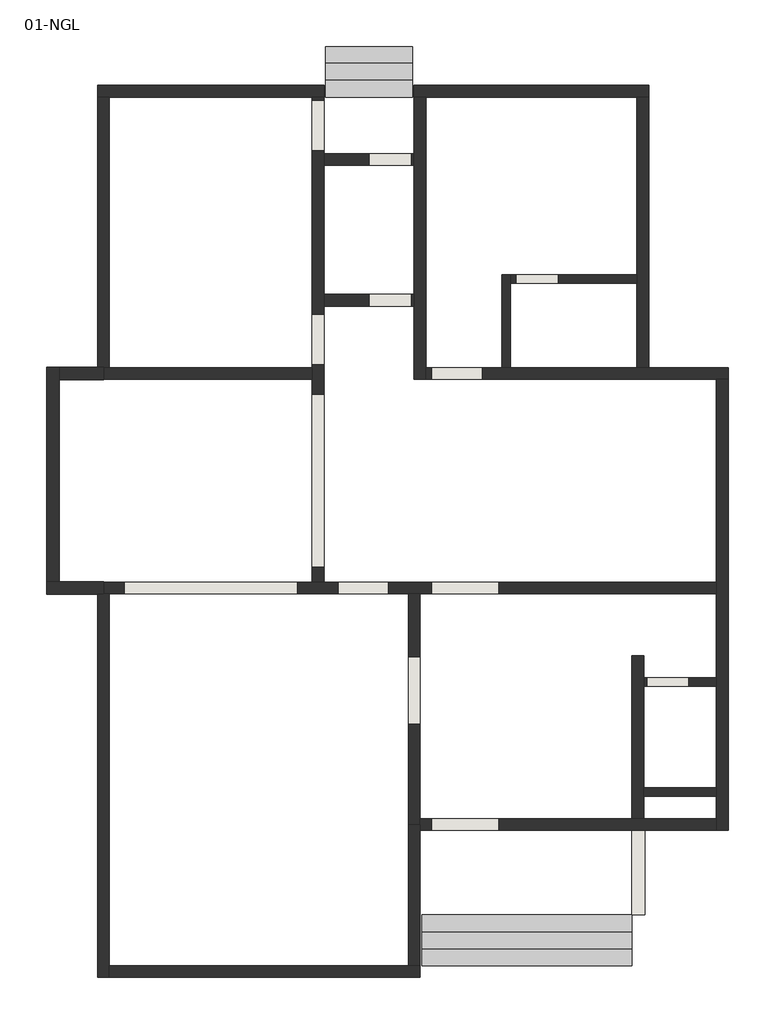
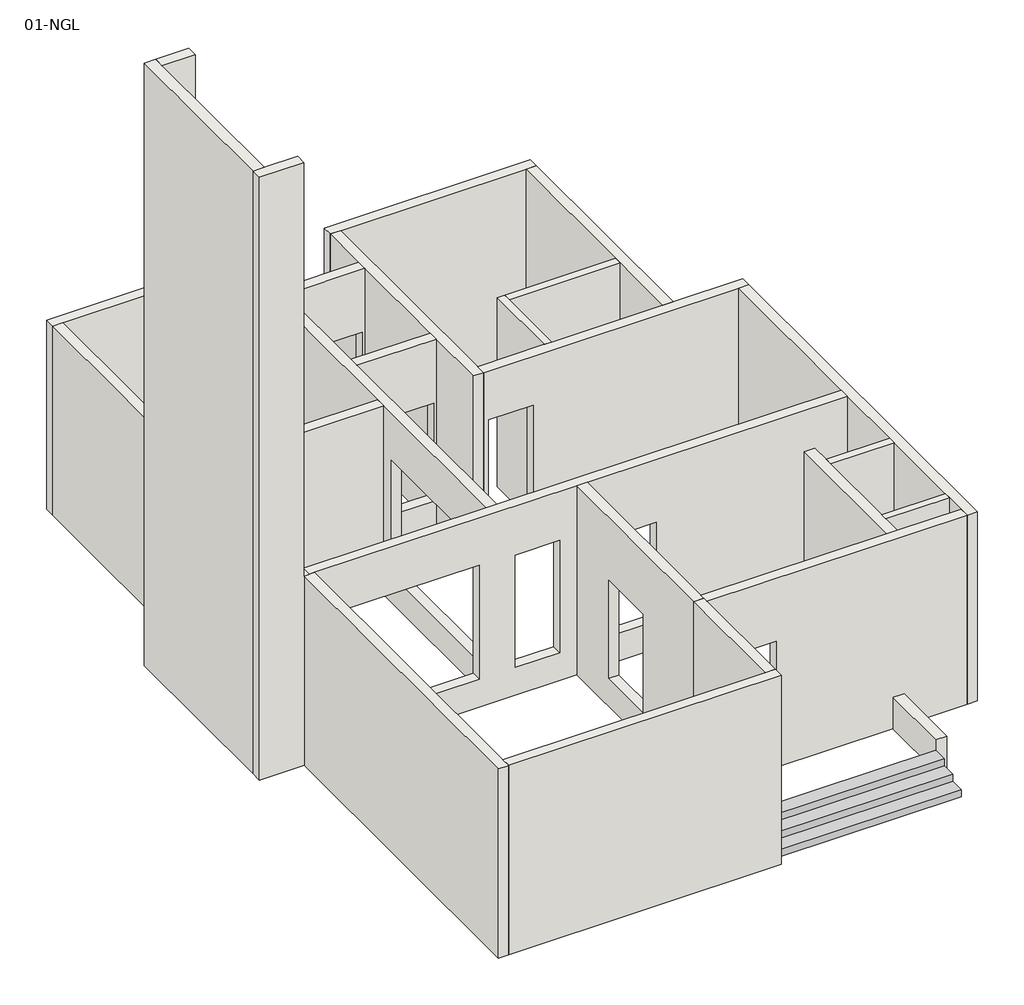
# One storey: 26 walls, 2 stair flights.
"""IFC4 building model written with IfcOpenShell, lengths in millimetres."""

from ifc_helpers import new_model, si_unit, frame, origin, origin_with_axes, place, context, project, spatial, polyline, outline, extrude, faceted_brep, element, save

model = new_model("IFC4")

# Units and contexts
model_context = context("Model", 3, world=origin())
ifc_project = project(units=[si_unit("LENGTHUNIT", "METRE", prefix="MILLI")], contexts=[model_context])

# Site, building, storey
site = spatial("IfcSite", under=ifc_project)
building = spatial("IfcBuilding", under=site)
storey = spatial("IfcBuildingStorey", under=building, Name="01-NGL", Elevation=0.0)

# Stair flights
placement = place(None, origin())
element("IfcStairFlight", 1, ObjectType="00-STEPS", at=placement, inside=storey, context=model_context, shape_type="Brep", body=[
    faceted_brep([(-8789.1107921, -18814.8987034, 150.0), (-8789.1107921, -19114.8987034, 150.0), (-5054.1107921, -19114.8987034, 150.0), (-5054.1107921, -18814.8987034, 150.0), (-8789.1107921, -18814.8987034, 0.0), (-8789.1107921, -19114.8987034, 0.0), (-5054.1107921, -19114.8987034, 0.0), (-5054.1107921, -18814.8987034, 0.0), (-8789.1107921, -18514.8987034, 300.0), (-8789.1107921, -18814.8987034, 300.0), (-5054.1107921, -18814.8987034, 300.0), (-5054.1107921, -18514.8987034, 300.0), (-8789.1107921, -18514.8987034, 0.0), (-5054.1107921, -18514.8987034, 0.0), (-8789.1107921, -18214.8987034, 0.0), (-5054.1107921, -18214.8987034, 0.0), (-8789.1107921, -18214.8987034, 450.0), (-8789.1107921, -18514.8987034, 450.0), (-5054.1107921, -18514.8987034, 450.0), (-5054.1107921, -18214.8987034, 450.0)], [[[0, 1, 2, 3]], [[1, 0, 4, 5]], [[2, 1, 5, 6]], [[3, 2, 6, 7]], [[8, 9, 10, 11]], [[4, 0, 9, 8, 12]], [[0, 3, 10, 9]], [[3, 7, 13, 11, 10]], [[5, 4, 12, 14, 15, 13, 7, 6]], [[16, 17, 18, 19]], [[12, 8, 17, 16, 14]], [[8, 11, 18, 17]], [[11, 13, 15, 19, 18]], [[16, 19, 15, 14]]]),
])
element("IfcStairFlight", 2, ObjectType="00-STEPS", at=placement, inside=storey, context=model_context, shape_type="Brep", body=[
    faceted_brep([(-8954.1107921, -3094.8987034, 150.0), (-8954.1107921, -2794.8987034, 150.0), (-10499.1107921, -2794.8987034, 150.0), (-10499.1107921, -3094.8987034, 150.0), (-8954.1107921, -3094.8987034, 0.0), (-8954.1107921, -2794.8987034, 0.0), (-10499.1107921, -2794.8987034, 0.0), (-10499.1107921, -3094.8987034, 0.0), (-8954.1107921, -3394.8987034, 300.0), (-8954.1107921, -3094.8987034, 300.0), (-10499.1107921, -3094.8987034, 300.0), (-10499.1107921, -3394.8987034, 300.0), (-8954.1107921, -3394.8987034, 0.0), (-10499.1107921, -3394.8987034, 0.0), (-8954.1107921, -3694.8987034, 0.0), (-10499.1107921, -3694.8987034, 0.0), (-8954.1107921, -3694.8987034, 450.0), (-8954.1107921, -3394.8987034, 450.0), (-10499.1107921, -3394.8987034, 450.0), (-10499.1107921, -3694.8987034, 450.0)], [[[0, 1, 2, 3]], [[1, 0, 4, 5]], [[2, 1, 5, 6]], [[3, 2, 6, 7]], [[8, 9, 10, 11]], [[4, 0, 9, 8, 12]], [[0, 3, 10, 9]], [[3, 7, 13, 11, 10]], [[5, 4, 12, 14, 15, 13, 7, 6]], [[16, 17, 18, 19]], [[12, 8, 17, 16, 14]], [[8, 11, 18, 17]], [[11, 13, 15, 19, 18]], [[16, 19, 15, 14]]]),
])

# Walls
element("IfcWall", 3, ObjectType="00 BRICK WALL", at=placement, inside=storey, context=model_context, shape_type="Brep", body=[
    faceted_brep([(-15456.6107921, -8487.3987034, 0.0), (-15456.6107921, -12297.3987034, 0.0), (-15456.6107921, -12297.3987034, 12900.0), (-15456.6107921, -8487.3987034, 12900.0), (-15231.6107921, -8487.3987034, 0.0), (-15231.6107921, -8487.3987034, 12900.0), (-15231.6107921, -8712.3987034, 12900.0), (-15231.6107921, -12297.3987034, 12900.0), (-15231.6107921, -12297.3987034, 0.0), (-15231.6107921, -8712.3987034, 0.0)], [[[0, 1, 2, 3]], [[4, 5, 6, 7, 8, 9]], [[1, 0, 4, 9, 8]], [[3, 2, 7, 6, 5]], [[0, 3, 5, 4]], [[2, 1, 8, 7]]]),
])
element("IfcWall", 4, ObjectType="00 BRICK WALL", at=placement, inside=storey, context=model_context, shape_type="Brep", body=[
    faceted_brep([(-14444.1107921, -12297.3987034, 4050.0), (-14444.1107921, -12297.3987034, 0.0), (-15231.6107921, -12297.3987034, 0.0), (-15456.6107921, -12297.3987034, 0.0), (-15456.6107921, -12297.3987034, 12900.0), (-15231.6107921, -12297.3987034, 12900.0), (-14556.6107921, -12297.3987034, 12900.0), (-14556.6107921, -12297.3987034, 4050.0), (-14444.1107921, -12522.3987034, 0.0), (-14444.1107921, -12522.3987034, 4050.0), (-14549.1107921, -12522.3987034, 4050.0), (-14556.6107921, -12522.3987034, 4050.0), (-14556.6107921, -12522.3987034, 7500.0), (-14556.6107921, -12522.3987034, 12900.0), (-15456.6107921, -12522.3987034, 12900.0), (-15456.6107921, -12522.3987034, 0.0), (-14549.1107921, -12522.3987034, 0.0), (-14444.1107921, -12304.8987034, 0.0), (-14444.1107921, -12514.8987034, 0.0), (-14444.1107921, -12304.8987034, 4050.0), (-14444.1107921, -12514.8987034, 4050.0), (-14556.6107921, -12299.8987034, 4050.0)], [[[0, 1, 2, 3, 4, 5, 6, 7]], [[8, 9, 10, 11, 12, 13, 14, 15, 16]], [[3, 2, 1, 17, 18, 8, 16, 15]], [[6, 5, 4, 14, 13]], [[4, 3, 15, 14]], [[0, 19, 20, 9, 8, 18, 17, 1]], [[7, 21, 11, 10, 9, 20, 19, 0]], [[6, 13, 12, 11, 21, 7]]]),
])
element("IfcWall", 5, ObjectType="00 BRICK WALL", at=placement, inside=storey, context=model_context, shape_type="Brep", body=[
    faceted_brep([(-14444.1107921, -8487.3987034, 0.0), (-14549.1107921, -8487.3987034, 0.0), (-15231.6107921, -8487.3987034, 0.0), (-15231.6107921, -8487.3987034, 12900.0), (-14556.6107921, -8487.3987034, 12900.0), (-14556.6107921, -8487.3987034, 4050.0), (-14549.1107921, -8487.3987034, 4050.0), (-14444.1107921, -8487.3987034, 4050.0), (-14444.1107921, -8712.3987034, 0.0), (-14444.1107921, -8712.3987034, 4050.0), (-14556.6107921, -8712.3987034, 4050.0), (-14556.6107921, -8712.3987034, 7575.0), (-14556.6107921, -8712.3987034, 12900.0), (-15231.6107921, -8712.3987034, 12900.0), (-15231.6107921, -8712.3987034, 0.0), (-14444.1107921, -8494.8987034, 0.0), (-14444.1107921, -8704.8987034, 0.0), (-14444.1107921, -8494.8987034, 4050.0), (-14444.1107921, -8704.8987034, 4050.0)], [[[0, 1, 2, 3, 4, 5, 6, 7]], [[8, 9, 10, 11, 12, 13, 14]], [[2, 1, 0, 15, 16, 8, 14]], [[4, 3, 13, 12]], [[3, 2, 14, 13]], [[0, 7, 17, 18, 9, 8, 16, 15]], [[5, 10, 9, 18, 17, 7, 6]], [[5, 4, 12, 11, 10]]]),
])
element("IfcWall", 6, ObjectType="01-150 WALL", at=placement, inside=storey, context=model_context, shape_type="SweptSolid", body=[
    extrude(outline(polyline([(-3554.1107921, -16104.8987034), (-4844.1107921, -16104.8987034), (-4844.1107921, -15954.8987034), (-3554.1107921, -15954.8987034), (-3554.1107921, -16104.8987034)])), origin_with_axes(), (0.0, 0.0, 1.0), 4050.0),
])
element("IfcWall", 7, ObjectType="01-150 WALL", at=placement, inside=storey, context=model_context, shape_type="SweptSolid", body=[
    extrude(outline(polyline([(0.0, -4844.1107921), (0.0, -3554.1107921), (4050.0, -3554.1107921), (4050.0, -4844.1107921), (0.0, -4844.1107921)]), holes=[polyline([(600.0, -4794.1107921), (2700.0, -4794.1107921), (2700.0, -4044.1107921), (600.0, -4044.1107921), (600.0, -4794.1107921)])]), frame((0.0, -14154.8987034, 0.0), z_axis=(0.0, 1.0, 0.0), x_axis=(0.0, 0.0, 1.0)), (0.0, 0.0, 1.0), 150.0),
])
element("IfcWall", 8, ObjectType="01-150 WALL", at=placement, inside=storey, context=model_context, shape_type="Brep", body=[
    faceted_brep([(-7214.1107921, -8494.8987034, 0.0), (-7214.1107921, -6994.8987034, 0.0), (-7214.1107921, -6844.8987034, 0.0), (-7214.1107921, -6844.8987034, 4050.0), (-7214.1107921, -6994.8987034, 4050.0), (-7214.1107921, -8494.8987034, 4050.0), (-7364.1107921, -8494.8987034, 0.0), (-7364.1107921, -8494.8987034, 4050.0), (-7364.1107921, -6844.8987034, 4050.0), (-7364.1107921, -6844.8987034, 0.0)], [[[0, 1, 2, 3, 4, 5]], [[6, 7, 8, 9]], [[2, 1, 0, 6, 9]], [[5, 4, 3, 8, 7]], [[0, 5, 7, 6]], [[3, 2, 9, 8]]]),
])
element("IfcWall", 9, ObjectType="01-150 WALL", at=placement, inside=storey, context=model_context, shape_type="SweptSolid", body=[
    extrude(outline(polyline([(0.0, -7214.1107921), (0.0, -4964.1107921), (4050.0, -4964.1107921), (4050.0, -7214.1107921), (0.0, -7214.1107921)]), holes=[polyline([(600.0, -7114.1107921), (2700.0, -7114.1107921), (2700.0, -6364.1107921), (600.0, -6364.1107921), (600.0, -7114.1107921)])]), frame((0.0, -6994.8987034, 0.0), z_axis=(0.0, 1.0, 0.0), x_axis=(0.0, 0.0, 1.0)), (0.0, 0.0, 1.0), 150.0),
])
element("IfcWall", 10, ObjectType="01-225 WALL", at=placement, inside=storey, context=model_context, shape_type="SweptSolid", body=[
    extrude(outline(polyline([(-4829.1107921, -16714.8987034), (-4829.1107921, -18214.8987034), (-5054.1107921, -18214.8987034), (-5054.1107921, -16714.8987034), (-4829.1107921, -16714.8987034)])), origin_with_axes(), (0.0, 0.0, 1.0), 675.0),
])
element("IfcWall", 11, ObjectType="01-225 WALL MAIN", at=placement, inside=storey, context=model_context, shape_type="Brep", body=[
    faceted_brep([(-4754.1107921, -8494.8987034, 0.0), (-4754.1107921, -3694.8987034, 0.0), (-4754.1107921, -3694.8987034, 4050.0), (-4754.1107921, -8494.8987034, 4050.0), (-4964.1107921, -8494.8987034, 0.0), (-4964.1107921, -8494.8987034, 4050.0), (-4964.1107921, -6994.8987034, 4050.0), (-4964.1107921, -6844.8987034, 4050.0), (-4964.1107921, -3694.8987034, 4050.0), (-4964.1107921, -3694.8987034, 0.0), (-4964.1107921, -6844.8987034, 0.0), (-4964.1107921, -6994.8987034, 0.0)], [[[0, 1, 2, 3]], [[4, 5, 6, 7, 8, 9, 10, 11]], [[1, 0, 4, 11, 10, 9]], [[3, 2, 8, 7, 6, 5]], [[2, 1, 9, 8]], [[0, 3, 5, 4]]]),
])
element("IfcWall", 12, ObjectType="01-225 WALL MAIN", at=placement, inside=storey, context=model_context, shape_type="Brep", body=[
    faceted_brep([(-8714.1107921, -8704.8987034, 0.0), (-8714.1107921, -8494.8987034, 0.0), (-8714.1107921, -3694.8987034, 0.0), (-8714.1107921, -3694.8987034, 4050.0), (-8714.1107921, -8494.8987034, 4050.0), (-8714.1107921, -8704.8987034, 4050.0), (-8924.1107921, -8704.8987034, 0.0), (-8924.1107921, -8704.8987034, 4050.0), (-8924.1107921, -7404.8987034, 4050.0), (-8924.1107921, -7194.8987034, 4050.0), (-8924.1107921, -4904.8987034, 4050.0), (-8924.1107921, -4694.8987034, 4050.0), (-8924.1107921, -3694.8987034, 4050.0), (-8924.1107921, -3694.8987034, 0.0), (-8924.1107921, -4694.8987034, 0.0), (-8924.1107921, -4904.8987034, 0.0), (-8924.1107921, -7194.8987034, 0.0), (-8924.1107921, -7404.8987034, 0.0)], [[[0, 1, 2, 3, 4, 5]], [[6, 7, 8, 9, 10, 11, 12, 13, 14, 15, 16, 17]], [[2, 1, 0, 6, 17, 16, 15, 14, 13]], [[5, 4, 3, 12, 11, 10, 9, 8, 7]], [[3, 2, 13, 12]], [[0, 5, 7, 6]]]),
])
element("IfcWall", 13, ObjectType="01-225 WALL MAIN", at=placement, inside=storey, context=model_context, shape_type="SweptSolid", body=[
    extrude(outline(polyline([(0.0, -10529.1107921), (0.0, -8924.1107921), (4050.0, -8924.1107921), (4050.0, -10529.1107921), (0.0, -10529.1107921)]), holes=[polyline([(2700.0, -8974.1107921), (600.0, -8974.1107921), (600.0, -9724.1107921), (2700.0, -9724.1107921), (2700.0, -8974.1107921)])]), frame((0.0, -4904.8987034, 0.0), z_axis=(0.0, 1.0, 0.0), x_axis=(0.0, 0.0, 1.0)), (0.0, 0.0, 1.0), 210.0),
])
element("IfcWall", 14, ObjectType="01-225 WALL MAIN", at=placement, inside=storey, context=model_context, shape_type="Brep", body=[
    faceted_brep([(-4754.1107921, -3484.8987034, 0.0), (-8924.1107921, -3484.8987034, 0.0), (-8924.1107921, -3484.8987034, 4050.0), (-4754.1107921, -3484.8987034, 4050.0), (-4754.1107921, -3694.8987034, 0.0), (-4754.1107921, -3694.8987034, 4050.0), (-4964.1107921, -3694.8987034, 4050.0), (-8714.1107921, -3694.8987034, 4050.0), (-8924.1107921, -3694.8987034, 4050.0), (-8924.1107921, -3694.8987034, 0.0), (-8714.1107921, -3694.8987034, 0.0), (-4964.1107921, -3694.8987034, 0.0)], [[[0, 1, 2, 3]], [[4, 5, 6, 7, 8, 9, 10, 11]], [[1, 0, 4, 11, 10, 9]], [[3, 2, 8, 7, 6, 5]], [[0, 3, 5, 4]], [[2, 1, 9, 8]]]),
])
element("IfcWall", 15, ObjectType="01-225 WALL MAIN", at=placement, inside=storey, context=model_context, shape_type="Brep", body=[
    faceted_brep([(-10529.1107921, -12304.8987034, 0.0), (-10529.1107921, -7404.8987034, 0.0), (-10529.1107921, -7194.8987034, 0.0), (-10529.1107921, -4904.8987034, 0.0), (-10529.1107921, -4694.8987034, 0.0), (-10529.1107921, -3694.8987034, 0.0), (-10529.1107921, -3694.8987034, 4050.0), (-10529.1107921, -4694.8987034, 4050.0), (-10529.1107921, -4904.8987034, 4050.0), (-10529.1107921, -7194.8987034, 4050.0), (-10529.1107921, -7404.8987034, 4050.0), (-10529.1107921, -12304.8987034, 4050.0), (-10529.1107921, -3744.8987034, 3000.0), (-10529.1107921, -3744.8987034, 600.0), (-10529.1107921, -4644.8987034, 600.0), (-10529.1107921, -4644.8987034, 3000.0), (-10529.1107921, -8444.8987034, 600.0), (-10529.1107921, -8444.8987034, 3000.0), (-10529.1107921, -7544.8987034, 3000.0), (-10529.1107921, -7544.8987034, 600.0), (-10529.1107921, -12044.8987034, 600.0), (-10529.1107921, -12044.8987034, 3040.0), (-10529.1107921, -8964.8987034, 3040.0), (-10529.1107921, -8964.8987034, 600.0), (-10739.1107921, -3694.8987034, 0.0), (-10739.1107921, -8494.8987034, 0.0), (-10739.1107921, -8704.8987034, 0.0), (-10739.1107921, -12304.8987034, 0.0), (-10739.1107921, -12304.8987034, 4050.0), (-10739.1107921, -8704.8987034, 4050.0), (-10739.1107921, -8494.8987034, 4050.0), (-10739.1107921, -3694.8987034, 4050.0), (-10739.1107921, -3744.8987034, 600.0), (-10739.1107921, -3744.8987034, 3000.0), (-10739.1107921, -4644.8987034, 3000.0), (-10739.1107921, -4644.8987034, 600.0), (-10739.1107921, -8444.8987034, 3000.0), (-10739.1107921, -8444.8987034, 600.0), (-10739.1107921, -7544.8987034, 600.0), (-10739.1107921, -7544.8987034, 3000.0), (-10739.1107921, -12044.8987034, 3040.0), (-10739.1107921, -12044.8987034, 600.0), (-10739.1107921, -8964.8987034, 600.0), (-10739.1107921, -8964.8987034, 3040.0)], [[[0, 1, 2, 3, 4, 5, 6, 7, 8, 9, 10, 11], [12, 13, 14, 15], [16, 17, 18, 19], [20, 21, 22, 23]], [[24, 25, 26, 27, 28, 29, 30, 31], [32, 33, 34, 35], [36, 37, 38, 39], [40, 41, 42, 43]], [[5, 4, 3, 2, 1, 0, 27, 26, 25, 24]], [[11, 10, 9, 8, 7, 6, 31, 30, 29, 28]], [[6, 5, 24, 31]], [[0, 11, 28, 27]], [[32, 13, 12, 33]], [[33, 12, 15, 34]], [[34, 15, 14, 35]], [[13, 32, 35, 14]], [[16, 37, 36, 17]], [[17, 36, 39, 18]], [[38, 19, 18, 39]], [[37, 16, 19, 38]], [[20, 41, 40, 21]], [[21, 40, 43, 22]], [[42, 23, 22, 43]], [[41, 20, 23, 42]]]),
])
element("IfcWall", 16, ObjectType="01-225 WALL MAIN", at=placement, inside=storey, context=model_context, shape_type="SweptSolid", body=[
    extrude(outline(polyline([(-14549.1107921, -8487.3987034), (-14549.1107921, -3694.8987034), (-14339.1107921, -3694.8987034), (-14339.1107921, -8494.8987034), (-14444.1107921, -8494.8987034), (-14444.1107921, -8487.3987034), (-14549.1107921, -8487.3987034)])), origin_with_axes(), (0.0, 0.0, 1.0), 4050.0),
])
element("IfcWall", 17, ObjectType="01-225 WALL MAIN", at=placement, inside=storey, context=model_context, shape_type="Brep", body=[
    faceted_brep([(-14339.1107921, -19324.8987034, 4050.0), (-14339.1107921, -19324.8987034, 0.0), (-8819.1107921, -19324.8987034, 0.0), (-8819.1107921, -19324.8987034, 4050.0), (-14339.1107921, -19114.8987034, 0.0), (-14339.1107921, -19114.8987034, 4050.0), (-9029.1107921, -19114.8987034, 4050.0), (-8819.1107921, -19114.8987034, 4050.0), (-8819.1107921, -19114.8987034, 0.0), (-9029.1107921, -19114.8987034, 0.0)], [[[0, 1, 2, 3]], [[4, 5, 6, 7, 8, 9]], [[2, 1, 4, 9, 8]], [[0, 3, 7, 6, 5]], [[3, 2, 8, 7]], [[0, 5, 4, 1]]]),
])
element("IfcWall", 18, ObjectType="01-225 WALL MAIN", at=placement, inside=storey, context=model_context, shape_type="Brep", body=[
    faceted_brep([(-9029.1107921, -16609.8987034, 0.0), (-9029.1107921, -19114.8987034, 0.0), (-9029.1107921, -19114.8987034, 4050.0), (-9029.1107921, -16609.8987034, 4050.0), (-8819.1107921, -16609.8987034, 0.0), (-8819.1107921, -16609.8987034, 4050.0), (-8819.1107921, -16714.8987034, 4050.0), (-8819.1107921, -19114.8987034, 4050.0), (-8819.1107921, -19114.8987034, 0.0), (-8819.1107921, -16714.8987034, 0.0)], [[[0, 1, 2, 3]], [[4, 5, 6, 7, 8, 9]], [[1, 0, 4, 9, 8]], [[3, 2, 7, 6, 5]], [[0, 3, 5, 4]], [[2, 1, 8, 7]]]),
])
element("IfcWall", 19, ObjectType="01-225 WALL MAIN", at=placement, inside=storey, context=model_context, shape_type="Brep", body=[
    faceted_brep([(-9029.1107921, -12514.8987034, 0.0), (-9029.1107921, -16609.8987034, 0.0), (-9029.1107921, -16609.8987034, 4050.0), (-9029.1107921, -12514.8987034, 4050.0), (-9029.1107921, -13629.8987034, 600.0), (-9029.1107921, -13629.8987034, 2700.0), (-9029.1107921, -14829.8987034, 2700.0), (-9029.1107921, -14829.8987034, 600.0), (-8819.1107921, -16609.8987034, 0.0), (-8819.1107921, -16504.8987034, 0.0), (-8819.1107921, -12514.8987034, 0.0), (-8819.1107921, -12514.8987034, 4050.0), (-8819.1107921, -16504.8987034, 4050.0), (-8819.1107921, -16609.8987034, 4050.0), (-8819.1107921, -13629.8987034, 2700.0), (-8819.1107921, -13629.8987034, 600.0), (-8819.1107921, -14829.8987034, 600.0), (-8819.1107921, -14829.8987034, 2700.0)], [[[0, 1, 2, 3], [4, 5, 6, 7]], [[8, 9, 10, 11, 12, 13], [14, 15, 16, 17]], [[1, 0, 10, 9, 8]], [[2, 1, 8, 13]], [[3, 2, 13, 12, 11]], [[0, 3, 11, 10]], [[4, 15, 14, 5]], [[5, 14, 17, 6]], [[6, 17, 16, 7]], [[15, 4, 7, 16]]]),
])
element("IfcWall", 20, ObjectType="01-225 WALL MAIN", at=placement, inside=storey, context=model_context, shape_type="Brep", body=[
    faceted_brep([(-8819.1107921, -16714.8987034, 0.0), (-5054.1107921, -16714.8987034, 0.0), (-4829.1107921, -16714.8987034, 0.0), (-3554.1107921, -16714.8987034, 0.0), (-3554.1107921, -16714.8987034, 4050.0), (-8819.1107921, -16714.8987034, 4050.0), (-8619.1107921, -16714.8987034, 600.0), (-8619.1107921, -16714.8987034, 2700.0), (-7419.1107921, -16714.8987034, 2700.0), (-7419.1107921, -16714.8987034, 600.0), (-3554.1107921, -16504.8987034, 0.0), (-4844.1107921, -16504.8987034, 0.0), (-5054.1107921, -16504.8987034, 0.0), (-8819.1107921, -16504.8987034, 0.0), (-8819.1107921, -16504.8987034, 4050.0), (-5054.1107921, -16504.8987034, 4050.0), (-4844.1107921, -16504.8987034, 4050.0), (-3554.1107921, -16504.8987034, 4050.0), (-8619.1107921, -16504.8987034, 2700.0), (-8619.1107921, -16504.8987034, 600.0), (-7419.1107921, -16504.8987034, 600.0), (-7419.1107921, -16504.8987034, 2700.0), (-8819.1107921, -16609.8987034, 0.0), (-8819.1107921, -16609.8987034, 4050.0)], [[[0, 1, 2, 3, 4, 5], [6, 7, 8, 9]], [[10, 11, 12, 13, 14, 15, 16, 17], [18, 19, 20, 21]], [[3, 2, 1, 0, 22, 13, 12, 11, 10]], [[5, 4, 17, 16, 15, 14, 23]], [[0, 5, 23, 14, 13, 22]], [[4, 3, 10, 17]], [[6, 19, 18, 7]], [[7, 18, 21, 8]], [[8, 21, 20, 9]], [[19, 6, 9, 20]]]),
])
element("IfcWall", 21, ObjectType="01-225 WALL MAIN", at=placement, inside=storey, context=model_context, shape_type="Brep", body=[
    faceted_brep([(-3554.1107921, -8704.8987034, 0.0), (-3554.1107921, -12304.8987034, 0.0), (-3554.1107921, -12514.8987034, 0.0), (-3554.1107921, -14004.8987034, 0.0), (-3554.1107921, -14154.8987034, 0.0), (-3554.1107921, -15954.8987034, 0.0), (-3554.1107921, -16104.8987034, 0.0), (-3554.1107921, -16504.8987034, 0.0), (-3554.1107921, -16714.8987034, 0.0), (-3554.1107921, -16714.8987034, 4050.0), (-3554.1107921, -16504.8987034, 4050.0), (-3554.1107921, -16104.8987034, 4050.0), (-3554.1107921, -15954.8987034, 4050.0), (-3554.1107921, -14154.8987034, 4050.0), (-3554.1107921, -14004.8987034, 4050.0), (-3554.1107921, -12514.8987034, 4050.0), (-3554.1107921, -12304.8987034, 4050.0), (-3554.1107921, -8704.8987034, 4050.0), (-3344.1107921, -8704.8987034, 0.0), (-3344.1107921, -8704.8987034, 4050.0), (-3344.1107921, -16714.8987034, 4050.0), (-3344.1107921, -16714.8987034, 0.0)], [[[0, 1, 2, 3, 4, 5, 6, 7, 8, 9, 10, 11, 12, 13, 14, 15, 16, 17]], [[18, 19, 20, 21]], [[8, 7, 6, 5, 4, 3, 2, 1, 0, 18, 21]], [[17, 16, 15, 14, 13, 12, 11, 10, 9, 20, 19]], [[9, 8, 21, 20]], [[0, 17, 19, 18]]]),
])
element("IfcWall", 22, ObjectType="01-225 WALL MAIN", at=placement, inside=storey, context=model_context, shape_type="Brep", body=[
    faceted_brep([(-10529.1107921, -3484.8987034, 0.0), (-14549.1107921, -3484.8987034, 0.0), (-14549.1107921, -3484.8987034, 4050.0), (-10529.1107921, -3484.8987034, 4050.0), (-10529.1107921, -3694.8987034, 0.0), (-10529.1107921, -3694.8987034, 4050.0), (-10739.1107921, -3694.8987034, 4050.0), (-14339.1107921, -3694.8987034, 4050.0), (-14549.1107921, -3694.8987034, 4050.0), (-14549.1107921, -3694.8987034, 0.0), (-14339.1107921, -3694.8987034, 0.0), (-10739.1107921, -3694.8987034, 0.0)], [[[0, 1, 2, 3]], [[4, 5, 6, 7, 8, 9, 10, 11]], [[1, 0, 4, 11, 10, 9]], [[3, 2, 8, 7, 6, 5]], [[2, 1, 9, 8]], [[0, 3, 5, 4]]]),
])
element("IfcWall", 23, ObjectType="01-225 WALL MAIN", at=placement, inside=storey, context=model_context, shape_type="Brep", body=[
    faceted_brep([(-5054.1107921, -13609.8987034, 0.0), (-5054.1107921, -16504.8987034, 0.0), (-5054.1107921, -16504.8987034, 4050.0), (-5054.1107921, -13609.8987034, 4050.0), (-4844.1107921, -13609.8987034, 0.0), (-4844.1107921, -13609.8987034, 4050.0), (-4844.1107921, -14004.8987034, 4050.0), (-4844.1107921, -14154.8987034, 4050.0), (-4844.1107921, -15954.8987034, 4050.0), (-4844.1107921, -16104.8987034, 4050.0), (-4844.1107921, -16504.8987034, 4050.0), (-4844.1107921, -16504.8987034, 0.0), (-4844.1107921, -16104.8987034, 0.0), (-4844.1107921, -15954.8987034, 0.0), (-4844.1107921, -14154.8987034, 0.0), (-4844.1107921, -14004.8987034, 0.0)], [[[0, 1, 2, 3]], [[4, 5, 6, 7, 8, 9, 10, 11, 12, 13, 14, 15]], [[1, 0, 4, 15, 14, 13, 12, 11]], [[3, 2, 10, 9, 8, 7, 6, 5]], [[0, 3, 5, 4]], [[2, 1, 11, 10]]]),
])
element("IfcWall", 24, ObjectType="01-225 WALL MAIN", at=placement, inside=storey, context=model_context, shape_type="Brep", body=[
    faceted_brep([(-14549.1107921, -12522.3987034, 0.0), (-14549.1107921, -19324.8987034, 0.0), (-14549.1107921, -19324.8987034, 4050.0), (-14549.1107921, -12522.3987034, 4050.0), (-14339.1107921, -12514.8987034, 0.0), (-14339.1107921, -12514.8987034, 4050.0), (-14339.1107921, -19114.8987034, 4050.0), (-14339.1107921, -19324.8987034, 4050.0), (-14339.1107921, -19324.8987034, 0.0), (-14339.1107921, -19114.8987034, 0.0), (-14444.1107921, -12522.3987034, 0.0), (-14444.1107921, -12514.8987034, 0.0), (-14341.6107921, -19324.8987034, 4050.0), (-14444.1107921, -12514.8987034, 4050.0), (-14444.1107921, -12522.3987034, 4050.0)], [[[0, 1, 2, 3]], [[4, 5, 6, 7, 8, 9]], [[1, 0, 10, 11, 4, 9, 8]], [[3, 2, 12, 7, 6, 5, 13, 14]], [[0, 3, 14, 10]], [[14, 13, 11, 10]], [[13, 5, 4, 11]], [[1, 8, 7, 12, 2]]]),
])
element("IfcWall", 25, ObjectType="01-225 WALL MAIN", at=placement, inside=storey, context=model_context, shape_type="Brep", body=[
    faceted_brep([(-3344.1107921, -8494.8987034, 0.0), (-4754.1107921, -8494.8987034, 0.0), (-4964.1107921, -8494.8987034, 0.0), (-7214.1107921, -8494.8987034, 0.0), (-7364.1107921, -8494.8987034, 0.0), (-8714.1107921, -8494.8987034, 0.0), (-8714.1107921, -8494.8987034, 4050.0), (-7364.1107921, -8494.8987034, 4050.0), (-7214.1107921, -8494.8987034, 4050.0), (-4964.1107921, -8494.8987034, 4050.0), (-4754.1107921, -8494.8987034, 4050.0), (-3344.1107921, -8494.8987034, 4050.0), (-8614.1107921, -8494.8987034, 3000.0), (-8614.1107921, -8494.8987034, 600.0), (-7714.1107921, -8494.8987034, 600.0), (-7714.1107921, -8494.8987034, 3000.0), (-8714.1107921, -8704.8987034, 0.0), (-3554.1107921, -8704.8987034, 0.0), (-3344.1107921, -8704.8987034, 0.0), (-3344.1107921, -8704.8987034, 4050.0), (-3554.1107921, -8704.8987034, 4050.0), (-8714.1107921, -8704.8987034, 4050.0), (-8614.1107921, -8704.8987034, 600.0), (-8614.1107921, -8704.8987034, 3000.0), (-7714.1107921, -8704.8987034, 3000.0), (-7714.1107921, -8704.8987034, 600.0)], [[[0, 1, 2, 3, 4, 5, 6, 7, 8, 9, 10, 11], [12, 13, 14, 15]], [[16, 17, 18, 19, 20, 21], [22, 23, 24, 25]], [[5, 4, 3, 2, 1, 0, 18, 17, 16]], [[11, 10, 9, 8, 7, 6, 21, 20, 19]], [[0, 11, 19, 18]], [[6, 5, 16, 21]], [[22, 13, 12, 23]], [[23, 12, 15, 24]], [[24, 15, 14, 25]], [[13, 22, 25, 14]]]),
])
element("IfcWall", 26, ObjectType="01-225 WALL MAIN", at=placement, inside=storey, context=model_context, shape_type="Brep", body=[
    faceted_brep([(-3554.1107921, -12304.8987034, 0.0), (-10529.1107921, -12304.8987034, 0.0), (-10739.1107921, -12304.8987034, 0.0), (-14444.1107921, -12304.8987034, 0.0), (-14444.1107921, -12304.8987034, 4050.0), (-10739.1107921, -12304.8987034, 4050.0), (-10529.1107921, -12304.8987034, 4050.0), (-3554.1107921, -12304.8987034, 4050.0), (-8619.1107921, -12304.8987034, 2700.0), (-8619.1107921, -12304.8987034, 600.0), (-7419.1107921, -12304.8987034, 600.0), (-7419.1107921, -12304.8987034, 2700.0), (-9379.1107921, -12304.8987034, 600.0), (-9379.1107921, -12304.8987034, 3000.0), (-10279.1107921, -12304.8987034, 3000.0), (-10279.1107921, -12304.8987034, 600.0), (-10999.1107921, -12304.8987034, 600.0), (-10999.1107921, -12304.8987034, 3040.0), (-14079.1107921, -12304.8987034, 3040.0), (-14079.1107921, -12304.8987034, 600.0), (-14444.1107921, -12514.8987034, 0.0), (-14339.1107921, -12514.8987034, 0.0), (-9029.1107921, -12514.8987034, 0.0), (-8819.1107921, -12514.8987034, 0.0), (-3554.1107921, -12514.8987034, 0.0), (-3554.1107921, -12514.8987034, 4050.0), (-8819.1107921, -12514.8987034, 4050.0), (-9029.1107921, -12514.8987034, 4050.0), (-14339.1107921, -12514.8987034, 4050.0), (-14444.1107921, -12514.8987034, 4050.0), (-8619.1107921, -12514.8987034, 600.0), (-8619.1107921, -12514.8987034, 2700.0), (-7419.1107921, -12514.8987034, 2700.0), (-7419.1107921, -12514.8987034, 600.0), (-9379.1107921, -12514.8987034, 3000.0), (-9379.1107921, -12514.8987034, 600.0), (-10279.1107921, -12514.8987034, 600.0), (-10279.1107921, -12514.8987034, 3000.0), (-10999.1107921, -12514.8987034, 3040.0), (-10999.1107921, -12514.8987034, 600.0), (-14079.1107921, -12514.8987034, 600.0), (-14079.1107921, -12514.8987034, 3040.0)], [[[0, 1, 2, 3, 4, 5, 6, 7], [8, 9, 10, 11], [12, 13, 14, 15], [16, 17, 18, 19]], [[20, 21, 22, 23, 24, 25, 26, 27, 28, 29], [30, 31, 32, 33], [34, 35, 36, 37], [38, 39, 40, 41]], [[3, 2, 1, 0, 24, 23, 22, 21, 20]], [[4, 3, 20, 29]], [[7, 6, 5, 4, 29, 28, 27, 26, 25]], [[0, 7, 25, 24]], [[30, 9, 8, 31]], [[31, 8, 11, 32]], [[10, 33, 32, 11]], [[9, 30, 33, 10]], [[12, 35, 34, 13]], [[13, 34, 37, 14]], [[36, 15, 14, 37]], [[35, 12, 15, 36]], [[16, 39, 38, 17]], [[17, 38, 41, 18]], [[18, 41, 40, 19]], [[39, 16, 19, 40]]]),
])
element("IfcWall", 27, ObjectType="01-225 WALL MAIN", at=placement, inside=storey, context=model_context, shape_type="SweptSolid", body=[
    extrude(outline(polyline([(0.0, -10529.1107921), (0.0, -8924.1107921), (4050.0, -8924.1107921), (4050.0, -10529.1107921), (0.0, -10529.1107921)]), holes=[polyline([(2700.0, -8974.1107921), (600.0, -8974.1107921), (600.0, -9724.1107921), (2700.0, -9724.1107921), (2700.0, -8974.1107921)])]), frame((0.0, -7404.8987034, 0.0), z_axis=(0.0, 1.0, 0.0), x_axis=(0.0, 0.0, 1.0)), (0.0, 0.0, 1.0), 210.0),
])
element("IfcWall", 28, ObjectType="01-225 WALL MAIN", at=placement, inside=storey, context=model_context, shape_type="Brep", body=[
    faceted_brep([(-10739.1107921, -8494.8987034, 0.0), (-14339.1107921, -8494.8987034, 0.0), (-14444.1107921, -8494.8987034, 0.0), (-14444.1107921, -8494.8987034, 4050.0), (-14339.1107921, -8494.8987034, 4050.0), (-10739.1107921, -8494.8987034, 4050.0), (-10739.1107921, -8704.8987034, 0.0), (-10739.1107921, -8704.8987034, 4050.0), (-14444.1107921, -8704.8987034, 4050.0), (-14444.1107921, -8704.8987034, 0.0)], [[[0, 1, 2, 3, 4, 5]], [[6, 7, 8, 9]], [[2, 1, 0, 6, 9]], [[3, 2, 9, 8]], [[5, 4, 3, 8, 7]], [[0, 5, 7, 6]]]),
])

save(model, "model.ifc")

# Revit data of these elements
# Type "00 BRICK WALL"
#   Type Mark = "G06"
#   Layers, outside or top first: 225 mm "MY STONE WALL" (function 1)
# Type "01-150 WALL"
#   Type Mark = "G06"
#   Layers, outside or top first: 150 mm "MY WHITE WALL PAINT" (function 1)
# Type "01-225 WALL"
#   Type Mark = "G06"
#   Layers, outside or top first: 225 mm "MY WHITE WALL PAINT" (function 1)
# Type "01-225 WALL MAIN"
#   Description = "Generic Wall (Material By Category), 200mm thick"
#   Assembly Code = "B2010"
#   Type Mark = "G06"
#   Layers, outside or top first: 5 mm "01-WHITE WALL PAINT" (function 4); 200 mm "01-DEFAULT WALL" (function 1); 5 mm "01-WHITE WALL PAINT" (function 5)
# Elements 1, 2 (IfcStairFlight, "00-STEPS")
#   Phase Created = New Construction
#   Materials on its faces: "01-FLOOR SLAB"
# Elements 3, 4, 5 (IfcWall, "00 BRICK WALL")
#   Top Offset = 0 mm
#   Base Offset = 0 mm
#   wall height = 12900 mm
#   Phase Created = New Construction
#   Base Constraint = 01-NGL
#   Top Constraint = 10-PARAPET LEVEL
#   Materials on its faces: "MY STONE WALL"
# Elements 6, 7, 8, 9 (IfcWall, "01-150 WALL")
#   Top Offset = 0 mm
#   Base Offset = 0 mm
#   wall height = 4050 mm
#   Phase Created = New Construction
#   Base Constraint = 01-NGL
#   Top Constraint = 04-FIRST FLOOR
#   Materials on its faces: "MY WHITE WALL PAINT"
# Element 10 (IfcWall, "01-225 WALL")
#   Top Offset = 75 mm
#   Base Offset = 0 mm
#   wall height = 675 mm
#   Phase Created = New Construction
#   Base Constraint = 01-NGL
#   Top Constraint = 02-DPC
#   Materials on its faces: "MY WHITE WALL PAINT"
# Elements 11, 13, 15, 16, 18, 19, 20, 23, 24, 25, 26, 27, 28 (IfcWall, "01-225 WALL MAIN")
#   Top Offset = 0 mm
#   Base Offset = 0 mm
#   wall height = 4050 mm
#   Phase Created = New Construction
#   Base Constraint = 01-NGL
#   Top Constraint = 04-FIRST FLOOR
#   Materials on its faces: "Default Wall", "01-WHITE WALL PAINT"
# Elements 12, 14, 17, 21, 22 (IfcWall, "01-225 WALL MAIN")
#   Top Offset = 0 mm
#   Base Offset = 0 mm
#   wall height = 4050 mm
#   Phase Created = New Construction
#   Base Constraint = 01-NGL
#   Top Constraint = 04-FIRST FLOOR
#   Materials on its faces: "01-WHITE WALL PAINT", "Default Wall"
# Materials
#   "MY STONE WALL": class "Gas", colour RGB 144 113 70, transparency 0, Description = "Air", Cost = 0
#   "MY WHITE WALL PAINT": class "Gas", colour RGB 0 0 0, transparency 0, Description = "Air", Cost = 0
#   "01-WHITE WALL PAINT": class "Generic", colour RGB 0 0 0, transparency 0, Description = "Acoustic Ceiling Tile 24 x 48", Cost = 0
#   "01-DEFAULT WALL": class "Generic", colour RGB 242 242 255, transparency 0, Description = "Acoustic Ceiling Tile 24 x 48", Cost = 0
#   "01-FLOOR SLAB": class "Generic", colour RGB 127 127 127, transparency 0, Description = "Acoustic Ceiling Tile 24 x 48", Cost = 0
#   "Default Wall": colour RGB 128 128 128, transparency 0, Cost = 0, Export to IFC = 0
